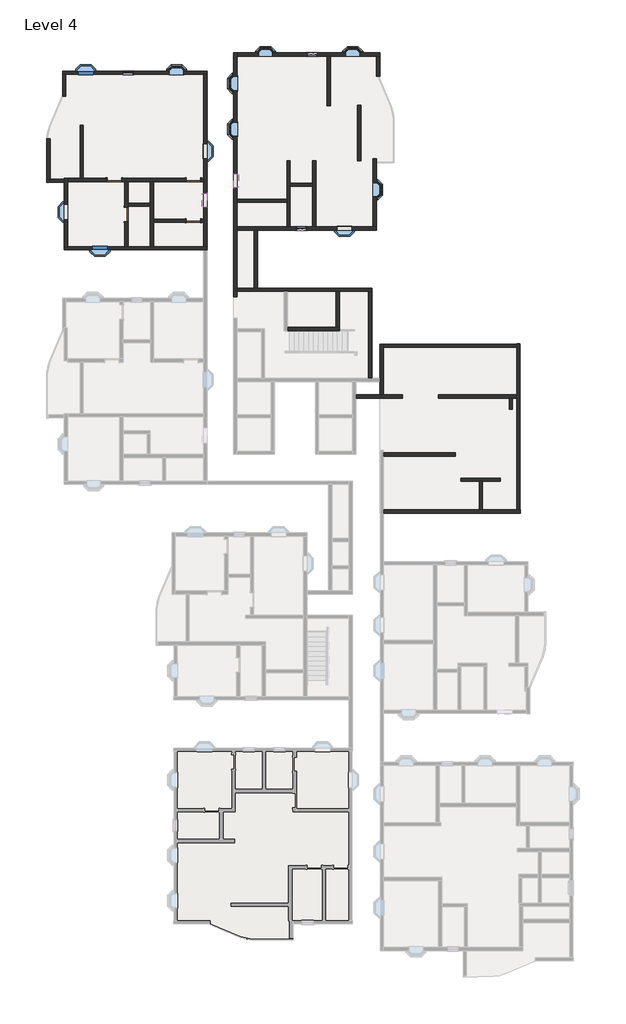
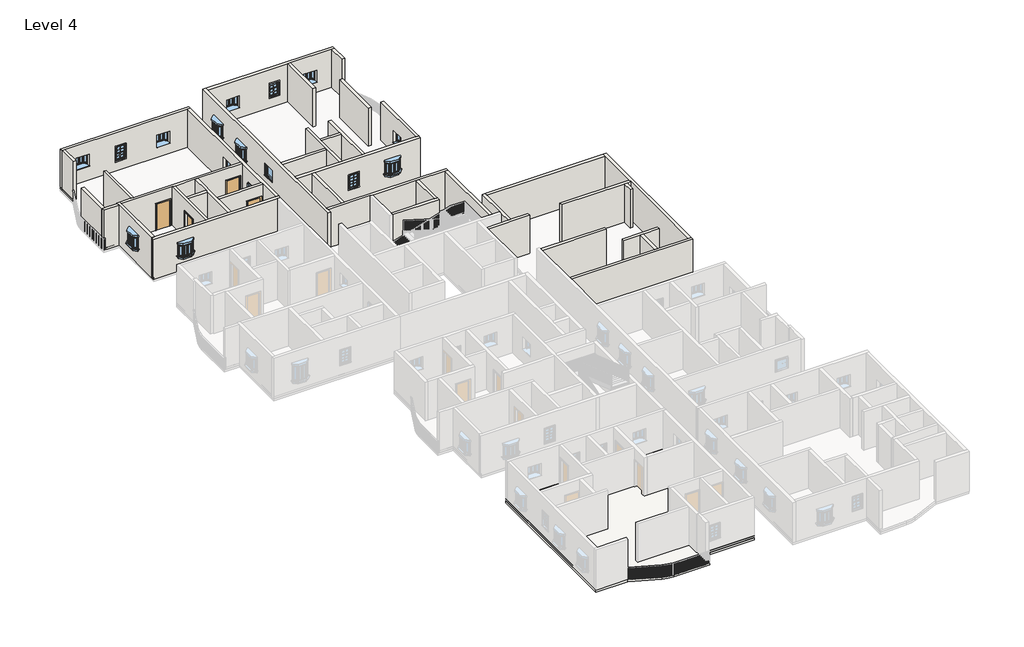
# One storey, part 4 of 14: 39 walls, 16 windows, 4 doors, 1 roof, 1 slab.
"""IFC4 building model written with IfcOpenShell, lengths in millimetres."""

from ifc_helpers import new_model, si_unit, point, frame, frame_2d, origin, place, context, project, spatial, polyline, circle_curve, trimmed, segment, composite_curve, outline, extrude, faceted_brep, transform, mapped, element, save
from components import door_719f80de, window_910x910mm_67ef725a, window_8debb0fa, windows_sgl_w_glazing_bars_910x910mm_256712d0

model = new_model("IFC4")

# Units and contexts
model_context = context("Model", 3, world=origin())
ifc_project = project(units=[si_unit("LENGTHUNIT", "METRE", prefix="MILLI")], contexts=[model_context])

# Site, building, storey
site = spatial("IfcSite", under=ifc_project)
building = spatial("IfcBuilding", under=site)
storey = spatial("IfcBuildingStorey", under=building, Name="Level 4", Elevation=9144.0)

# Doors
placement = place(None, origin())
door_shape = door_719f80de(model_context)
element("IfcDoor", 1, ObjectType="Single-Flush : 36\" x 84\"", at=placement, inside=storey, context=model_context, shape_type="MappedRepresentation", body=[
    mapped(door_shape, transform((-16068.1391351, 22048.4083494, 9144.0), x_axis=(1.0, 0.0, 0.0), y_axis=(0.0, 1.0, 0.0), z_axis=(0.0, 0.0, 1.0))),
])
element("IfcDoor", 2, ObjectType="Single-Flush : 36\" x 84\"", at=placement, inside=storey, context=model_context, shape_type="MappedRepresentation", body=[
    mapped(door_shape, transform((-15306.1391351, 19864.0083494, 9144.0), x_axis=(0.0, 1.0, 0.0), y_axis=(-1.0, 0.0, 0.0), z_axis=(0.0, 0.0, 1.0))),
])
element("IfcDoor", 3, ObjectType="Single-Flush : 36\" x 84\"", at=placement, inside=storey, context=model_context, shape_type="MappedRepresentation", body=[
    mapped(door_shape, transform((-11057.9891351, 19470.3083494, 9144.0), x_axis=(1.0, 0.0, 0.0), y_axis=(0.0, 1.0, 0.0), z_axis=(0.0, 0.0, 1.0))),
])
element("IfcDoor", 4, ObjectType="Single-Flush : 36\" x 84\"", at=placement, inside=storey, context=model_context, shape_type="MappedRepresentation", body=[
    mapped(door_shape, transform((-11057.9891351, 22048.4083494, 9144.0), x_axis=(1.0, 0.0, 0.0), y_axis=(0.0, 1.0, 0.0), z_axis=(0.0, 0.0, 1.0))),
])

# Roof
element("IfcRoof", 5, ObjectType="Generic - 12\"", at=placement, inside=storey, context=model_context, shape_type="SweptSolid", body=[
    extrude(outline(composite_curve([segment(polyline([(-10024.8708389, -25100.3416506), (-12290.487215, -25100.3416506), (-12290.487215, -13962.4416506), (-986.8891351, -13962.4416506), (-986.8891351, -25100.3416506), (-4746.0891351, -25100.3416506), (-4746.0891351, -26090.9416506), (-7315.6413127, -26090.9416506)]), True, "CONTINUOUS"), segment(trimmed(circle_curve(frame_2d((-7315.6413127, -24160.5416506)), 1930.4), [point((-7315.6413127, -26090.9416506))], [point((-8075.5356374, -25935.0851906))], False, "CARTESIAN"), True, "CONTINUOUS"), segment(polyline([(-8075.5356374, -25935.0851906), (-10024.8708389, -25100.3416506)]), True, "CONTINUOUS")], self_intersect=False)), frame((0.0, 0.0, 9144.0), z_axis=(0.0, 0.0, 1.0), x_axis=(1.0, 0.0, 0.0)), (0.0, 0.0, 1.0), 152.4),
])

# Slab
element("IfcSlab", 6, ObjectType="Generic - 12\"", at=placement, inside=storey, context=model_context, shape_type="SweptSolid", body=[
    extrude(outline(composite_curve([segment(polyline([(-10024.8708389, -25100.3416506), (-12290.487215, -25100.3416506), (-12290.487215, -13962.4416506), (-986.8891351, -13962.4416506), (-986.8891351, -25100.3416506), (-4746.0891351, -25100.3416506), (-4746.0891351, -26090.9416506), (-7315.6413127, -26090.9416506)]), True, "CONTINUOUS"), segment(trimmed(circle_curve(frame_2d((-7315.6413127, -24160.5416506)), 1930.4), [point((-7315.6413127, -26090.9416506))], [point((-8075.5356374, -25935.0851906))], False, "CARTESIAN"), True, "CONTINUOUS"), segment(polyline([(-8075.5356374, -25935.0851906), (-10024.8708389, -25100.3416506)]), True, "CONTINUOUS")], self_intersect=False)), frame((0.0, 0.0, 8991.6), z_axis=(0.0, 0.0, 1.0), x_axis=(1.0, 0.0, 0.0)), (0.0, 0.0, 1.0), 152.4),
])

# Walls
element("IfcWall", 7, ObjectType="4.5\" p", at=placement, inside=storey, context=model_context, shape_type="Brep", body=[
    faceted_brep([(-10600.7891351, 21946.8083494, 11277.6), (-10600.7891351, 21946.8083494, 9144.0), (-10397.5891351, 21946.8083494, 9144.0), (-10397.5891351, 21946.8083494, 12192.0), (-13578.9391351, 21946.8083494, 12192.0), (-13782.1391351, 21946.8083494, 12192.0), (-15204.5391351, 21946.8083494, 12192.0), (-15407.7391351, 21946.8083494, 12192.0), (-19033.5891351, 21946.8083494, 12192.0), (-19033.5891351, 21946.8083494, 9144.0), (-16525.3391351, 21946.8083494, 9144.0), (-16525.3391351, 21946.8083494, 11277.6), (-15610.9391351, 21946.8083494, 11277.6), (-15610.9391351, 21946.8083494, 9144.0), (-15407.7391351, 21946.8083494, 9144.0), (-15204.5391351, 21946.8083494, 9144.0), (-13782.1391351, 21946.8083494, 9144.0), (-13578.9391351, 21946.8083494, 9144.0), (-11515.1891351, 21946.8083494, 9144.0), (-11515.1891351, 21946.8083494, 11277.6), (-10397.5891351, 22150.0083494, 9144.0), (-10600.7891351, 22150.0083494, 9144.0), (-10600.7891351, 22150.0083494, 11277.6), (-11515.1891351, 22150.0083494, 11277.6), (-11515.1891351, 22150.0083494, 9144.0), (-15610.9391351, 22150.0083494, 9144.0), (-15610.9391351, 22150.0083494, 11277.6), (-16525.3391351, 22150.0083494, 11277.6), (-16525.3391351, 22150.0083494, 9144.0), (-18042.9891351, 22150.0083494, 9144.0), (-18246.1891351, 22150.0083494, 9144.0), (-19033.5891351, 22150.0083494, 9144.0), (-19033.5891351, 22150.0083494, 12192.0), (-18246.1891351, 22150.0083494, 12192.0), (-18042.9891351, 22150.0083494, 12192.0), (-10397.5891351, 22150.0083494, 12192.0)], [[[0, 1, 2, 3, 4, 5, 6, 7, 8, 9, 10, 11, 12, 13, 14, 15, 16, 17, 18, 19]], [[20, 21, 22, 23, 24, 25, 26, 27, 28, 29, 30, 31, 32, 33, 34, 35]], [[10, 9, 31, 30, 29, 28]], [[2, 1, 21, 20]], [[18, 17, 16, 15, 14, 13, 25, 24]], [[8, 7, 6, 5, 4, 3, 35, 34, 33, 32]], [[9, 8, 32, 31]], [[26, 25, 13, 12]], [[27, 26, 12, 11]], [[28, 27, 11, 10]], [[22, 21, 1, 0]], [[23, 22, 0, 19]], [[24, 23, 19, 18]], [[3, 2, 20, 35]]]),
])
element("IfcWall", 8, ObjectType="4.5\" p", at=placement, inside=storey, context=model_context, shape_type="Brep", body=[
    faceted_brep([(-15407.7391351, 21946.8083494, 9144.0), (-15407.7391351, 20321.2083494, 9144.0), (-15407.7391351, 20321.2083494, 11277.6), (-15407.7391351, 19406.8083494, 11277.6), (-15407.7391351, 19406.8083494, 9144.0), (-15407.7391351, 17812.9583494, 9144.0), (-15407.7391351, 17812.9583494, 12192.0), (-15407.7391351, 21946.8083494, 12192.0), (-15204.5391351, 20321.2083494, 11277.6), (-15204.5391351, 20321.2083494, 9144.0), (-15204.5391351, 20372.0083494, 9144.0), (-15204.5391351, 20575.2083494, 9144.0), (-15204.5391351, 21946.8083494, 9144.0), (-15204.5391351, 21946.8083494, 12192.0), (-15204.5391351, 20575.2083494, 12192.0), (-15204.5391351, 20372.0083494, 12192.0), (-15204.5391351, 17812.9583494, 12192.0), (-15204.5391351, 17812.9583494, 9144.0), (-15204.5391351, 19406.8083494, 9144.0), (-15204.5391351, 19406.8083494, 11277.6)], [[[0, 1, 2, 3, 4, 5, 6, 7]], [[8, 9, 10, 11, 12, 13, 14, 15, 16, 17, 18, 19]], [[18, 17, 5, 4]], [[12, 11, 10, 9, 1, 0]], [[7, 6, 16, 15, 14, 13]], [[6, 5, 17, 16]], [[0, 7, 13, 12]], [[2, 1, 9, 8]], [[3, 2, 8, 19]], [[4, 3, 19, 18]]]),
])
element("IfcWall", 9, ObjectType="4.5\" p", at=placement, inside=storey, context=model_context, shape_type="Brep", body=[
    faceted_brep([(-13782.1391351, 21946.8083494, 9144.0), (-13782.1391351, 20575.2083494, 9144.0), (-13782.1391351, 20372.0083494, 9144.0), (-13782.1391351, 17812.9583494, 9144.0), (-13782.1391351, 17812.9583494, 12192.0), (-13782.1391351, 20372.0083494, 12192.0), (-13782.1391351, 20575.2083494, 12192.0), (-13782.1391351, 21946.8083494, 12192.0), (-13578.9391351, 21946.8083494, 9144.0), (-13578.9391351, 21946.8083494, 12192.0), (-13578.9391351, 19571.9083494, 12192.0), (-13578.9391351, 19368.7083494, 12192.0), (-13578.9391351, 17812.9583494, 12192.0), (-13578.9391351, 17812.9583494, 9144.0), (-13578.9391351, 19368.7083494, 9144.0), (-13578.9391351, 19571.9083494, 9144.0)], [[[0, 1, 2, 3, 4, 5, 6, 7]], [[8, 9, 10, 11, 12, 13, 14, 15]], [[3, 2, 1, 0, 8, 15, 14, 13]], [[7, 6, 5, 4, 12, 11, 10, 9]], [[4, 3, 13, 12]], [[0, 7, 9, 8]]]),
])
element("IfcWall", 10, ObjectType="4.5\" p", at=placement, inside=storey, context=model_context, shape_type="SweptSolid", body=[
    extrude(outline(polyline([(-13782.1391351, 20372.0083494), (-15204.5391351, 20372.0083494), (-15204.5391351, 20575.2083494), (-13782.1391351, 20575.2083494), (-13782.1391351, 20372.0083494)])), frame((0.0, 0.0, 9144.0), z_axis=(0.0, 0.0, 1.0), x_axis=(1.0, 0.0, 0.0)), (0.0, 0.0, 1.0), 3048.0),
])
element("IfcWall", 11, ObjectType="4.5\" p", at=placement, inside=storey, context=model_context, shape_type="SweptSolid", body=[
    extrude(outline(polyline([(11277.6, -10600.7891351), (9144.0, -10600.7891351), (9144.0, -10397.5891351), (12192.0, -10397.5891351), (12192.0, -13578.9391351), (9144.0, -13578.9391351), (9144.0, -11515.1891351), (11277.6, -11515.1891351), (11277.6, -10600.7891351)])), frame((0.0, 19368.7083494, 0.0), z_axis=(0.0, 1.0, 0.0), x_axis=(0.0, 0.0, 1.0)), (0.0, 0.0, 1.0), 203.2),
])
element("IfcWall", 12, ObjectType="4.5\" p", at=placement, inside=storey, context=model_context, shape_type="SweptSolid", body=[
    extrude(outline(polyline([(-6993.9891351, 18875.1215905), (-6993.9891351, 15192.1215905), (-7197.1891351, 15192.1215905), (-7197.1891351, 18875.1215905), (-6993.9891351, 18875.1215905)])), frame((0.0, 0.0, 9144.0), z_axis=(0.0, 0.0, 1.0), x_axis=(1.0, 0.0, 0.0)), (0.0, 0.0, 1.0), 3048.0),
])
element("IfcWall", 13, ObjectType="4.5\" p", at=placement, inside=storey, context=model_context, shape_type="Brep", body=[
    faceted_brep([(-8289.3891351, 18875.1215905, 9144.0), (-7197.1891351, 18875.1215905, 9144.0), (-6993.9891351, 18875.1215905, 9144.0), (562.5108649, 18875.1215905, 9144.0), (562.5108649, 18875.1215905, 12192.0), (-6993.9891351, 18875.1215905, 12192.0), (-7197.1891351, 18875.1215905, 12192.0), (-8289.3891351, 18875.1215905, 12192.0), (-1017.6641351, 18875.1215905, 11254.0), (-1017.6641351, 18875.1215905, 10344.0), (-1927.6641351, 18875.1215905, 10344.0), (-1927.6641351, 18875.1215905, 11254.0), (-3876.1391351, 18875.1215905, 11125.2), (-3876.1391351, 18875.1215905, 10058.4), (-4536.5391351, 18875.1215905, 10058.4), (-4536.5391351, 18875.1215905, 11125.2), (-8289.3891351, 19078.3215905, 9144.0), (-8289.3891351, 19078.3215905, 12192.0), (-5120.7391351, 19078.3215905, 12192.0), (-4917.5391351, 19078.3215905, 12192.0), (-3495.1391351, 19078.3215905, 12192.0), (-3291.9391351, 19078.3215905, 12192.0), (346.6108649, 19078.3215905, 12192.0), (549.8108649, 19078.3215905, 12192.0), (562.5108649, 19078.3215905, 12192.0), (562.5108649, 19078.3215905, 9144.0), (549.8108649, 19078.3215905, 9144.0), (346.6108649, 19078.3215905, 9144.0), (-3291.9391351, 19078.3215905, 9144.0), (-3495.1391351, 19078.3215905, 9144.0), (-4917.5391351, 19078.3215905, 9144.0), (-5120.7391351, 19078.3215905, 9144.0), (-1017.6641351, 19078.3215905, 11254.0), (-1927.6641351, 19078.3215905, 11254.0), (-1927.6641351, 19078.3215905, 10344.0), (-1017.6641351, 19078.3215905, 10344.0), (-3876.1391351, 19078.3215905, 11125.2), (-4536.5391351, 19078.3215905, 11125.2), (-4536.5391351, 19078.3215905, 10058.4), (-3876.1391351, 19078.3215905, 10058.4)], [[[0, 1, 2, 3, 4, 5, 6, 7], [8, 9, 10, 11], [12, 13, 14, 15]], [[16, 17, 18, 19, 20, 21, 22, 23, 24, 25, 26, 27, 28, 29, 30, 31], [32, 33, 34, 35], [36, 37, 38, 39]], [[3, 2, 1, 0, 16, 31, 30, 29, 28, 27, 26, 25]], [[4, 3, 25, 24]], [[7, 6, 5, 4, 24, 23, 22, 21, 20, 19, 18, 17]], [[9, 8, 32, 35]], [[10, 9, 35, 34]], [[11, 10, 34, 33]], [[8, 11, 33, 32]], [[13, 12, 36, 39]], [[14, 13, 39, 38]], [[15, 14, 38, 37]], [[12, 15, 37, 36]], [[0, 7, 17, 16]]]),
])
element("IfcWall", 14, ObjectType="4.5\" p", at=placement, inside=storey, context=model_context, shape_type="SweptSolid", body=[
    extrude(outline(polyline([(19078.3215905, 9144.0), (19078.3215905, 12192.0), (23396.3215905, 12192.0), (23396.3215905, 9144.0), (19078.3215905, 9144.0)]), holes=[polyline([(21882.8215905, 10968.4), (20972.8215905, 10968.4), (20972.8215905, 10058.4), (21882.8215905, 10058.4), (21882.8215905, 10968.4)])]), frame((346.6108649, 0.0, 0.0), z_axis=(1.0, 0.0, 0.0), x_axis=(0.0, 1.0, 0.0)), (0.0, 0.0, 1.0), 203.2),
])
element("IfcWall", 15, ObjectType="4.5\" p", at=placement, inside=storey, context=model_context, shape_type="SweptSolid", body=[
    extrude(outline(polyline([(-5120.7391351, 20634.0715905), (-8289.3891351, 20634.0715905), (-8289.3891351, 20837.2715905), (-5120.7391351, 20837.2715905), (-5120.7391351, 20634.0715905)])), frame((0.0, 0.0, 9144.0), z_axis=(0.0, 0.0, 1.0), x_axis=(1.0, 0.0, 0.0)), (0.0, 0.0, 1.0), 3048.0),
])
element("IfcWall", 16, ObjectType="4.5\" p", at=placement, inside=storey, context=model_context, shape_type="Brep", body=[
    faceted_brep([(-5120.7391351, 23256.6215905, 9144.0), (-5120.7391351, 20837.2715905, 9144.0), (-5120.7391351, 20634.0715905, 9144.0), (-5120.7391351, 19078.3215905, 9144.0), (-5120.7391351, 19078.3215905, 12192.0), (-5120.7391351, 20634.0715905, 12192.0), (-5120.7391351, 20837.2715905, 12192.0), (-5120.7391351, 23256.6215905, 12192.0), (-4917.5391351, 23256.6215905, 9144.0), (-4917.5391351, 23256.6215905, 12192.0), (-4917.5391351, 21853.2715905, 12192.0), (-4917.5391351, 21650.0715905, 12192.0), (-4917.5391351, 19078.3215905, 12192.0), (-4917.5391351, 19078.3215905, 9144.0), (-4917.5391351, 21650.0715905, 9144.0), (-4917.5391351, 21853.2715905, 9144.0)], [[[0, 1, 2, 3, 4, 5, 6, 7]], [[8, 9, 10, 11, 12, 13, 14, 15]], [[3, 2, 1, 0, 8, 15, 14, 13]], [[7, 6, 5, 4, 12, 11, 10, 9]], [[0, 7, 9, 8]], [[4, 3, 13, 12]]]),
])
element("IfcWall", 17, ObjectType="4.5\" p", at=placement, inside=storey, context=model_context, shape_type="Brep", body=[
    faceted_brep([(-3495.1391351, 23256.6215905, 9144.0), (-3495.1391351, 21853.2715905, 9144.0), (-3495.1391351, 21650.0715905, 9144.0), (-3495.1391351, 19078.3215905, 9144.0), (-3495.1391351, 19078.3215905, 12192.0), (-3495.1391351, 21650.0715905, 12192.0), (-3495.1391351, 21853.2715905, 12192.0), (-3495.1391351, 23256.6215905, 12192.0), (-3291.9391351, 23256.6215905, 9144.0), (-3291.9391351, 23256.6215905, 12192.0), (-3291.9391351, 19078.3215905, 12192.0), (-3291.9391351, 19078.3215905, 9144.0)], [[[0, 1, 2, 3, 4, 5, 6, 7]], [[8, 9, 10, 11]], [[3, 2, 1, 0, 8, 11]], [[7, 6, 5, 4, 10, 9]], [[0, 7, 9, 8]], [[4, 3, 11, 10]]]),
])
element("IfcWall", 18, ObjectType="4.5\" p", at=placement, inside=storey, context=model_context, shape_type="SweptSolid", body=[
    extrude(outline(polyline([(-3495.1391351, 21650.0715905), (-4917.5391351, 21650.0715905), (-4917.5391351, 21853.2715905), (-3495.1391351, 21853.2715905), (-3495.1391351, 21650.0715905)])), frame((0.0, 0.0, 9144.0), z_axis=(0.0, 0.0, 1.0), x_axis=(1.0, 0.0, 0.0)), (0.0, 0.0, 1.0), 3048.0),
])
element("IfcWall", 19, ObjectType="4.5\" p", at=placement, inside=storey, context=model_context, shape_type="SweptSolid", body=[
    extrude(outline(polyline([(-1799.6891351, 14988.9215905), (-1799.6891351, 12709.2715905), (-2002.8891351, 12709.2715905), (-2002.8891351, 14988.9215905), (-1799.6891351, 14988.9215905)])), frame((0.0, 0.0, 9144.0), z_axis=(0.0, 0.0, 1.0), x_axis=(1.0, 0.0, 0.0)), (0.0, 0.0, 1.0), 3048.0),
])
element("IfcWall", 20, ObjectType="4.5\" p", at=placement, inside=storey, context=model_context, shape_type="Brep", body=[
    faceted_brep([(-5095.3391351, 12506.0715905, 9144.0), (-1786.9891351, 12506.0715905, 9144.0), (-1786.9891351, 12506.0715905, 12192.0), (-5095.3391351, 12506.0715905, 12192.0), (-5095.3391351, 12709.2715905, 9144.0), (-5095.3391351, 12709.2715905, 12192.0), (-2002.8891351, 12709.2715905, 12192.0), (-1799.6891351, 12709.2715905, 12192.0), (-1786.9891351, 12709.2715905, 12192.0), (-1786.9891351, 12709.2715905, 9144.0), (-1799.6891351, 12709.2715905, 9144.0), (-2002.8891351, 12709.2715905, 9144.0)], [[[0, 1, 2, 3]], [[4, 5, 6, 7, 8, 9, 10, 11]], [[1, 0, 4, 11, 10, 9]], [[2, 1, 9, 8]], [[3, 2, 8, 7, 6, 5]], [[0, 3, 5, 4]]]),
])
element("IfcWall", 21, ObjectType="4.5\" p", at=placement, inside=storey, context=model_context, shape_type="Brep", body=[
    faceted_brep([(-745.5891351, 8223.6457306, 9144.0), (2209.4205024, 8223.6457306, 9144.0), (2209.4205024, 8223.6457306, 12192.0), (-745.5891351, 8223.6457306, 12192.0), (-745.5891351, 8426.8457306, 9144.0), (-745.5891351, 8426.8457306, 12192.0), (793.5880523, 8426.8457306, 12192.0), (996.7880523, 8426.8457306, 12192.0), (2209.4205024, 8426.8457306, 12192.0), (2209.4205024, 8426.8457306, 9144.0), (996.7880523, 8426.8457306, 9144.0), (793.5880523, 8426.8457306, 9144.0)], [[[0, 1, 2, 3]], [[4, 5, 6, 7, 8, 9, 10, 11]], [[1, 0, 4, 11, 10, 9]], [[2, 1, 9, 8]], [[3, 2, 8, 7, 6, 5]], [[0, 3, 5, 4]]]),
])
element("IfcWall", 22, ObjectType="4.5\" p", at=placement, inside=storey, context=model_context, shape_type="Brep", body=[
    faceted_brep([(996.7880523, 8426.8457306, 9144.0), (996.7880523, 11443.0957306, 9144.0), (996.7880523, 11646.2957306, 9144.0), (996.7880523, 11646.2957306, 12192.0), (996.7880523, 11443.0957306, 12192.0), (996.7880523, 8426.8457306, 12192.0), (793.5880523, 8426.8457306, 9144.0), (793.5880523, 8426.8457306, 12192.0), (793.5880523, 9275.2949943, 12192.0), (793.5880523, 9478.4949943, 12192.0), (793.5880523, 11646.2957306, 12192.0), (793.5880523, 11646.2957306, 9144.0), (793.5880523, 9478.4949943, 9144.0), (793.5880523, 9275.2949943, 9144.0)], [[[0, 1, 2, 3, 4, 5]], [[6, 7, 8, 9, 10, 11, 12, 13]], [[2, 1, 0, 6, 13, 12, 11]], [[5, 4, 3, 10, 9, 8, 7]], [[0, 5, 7, 6]], [[3, 2, 11, 10]]]),
])
element("IfcWall", 23, ObjectType="4.5\" p", at=placement, inside=storey, context=model_context, shape_type="Brep", body=[
    faceted_brep([(9461.3380523, 8426.8457306, 9144.0), (4492.3034266, 8426.8457306, 9144.0), (4492.3034266, 8426.8457306, 12192.0), (9461.3380523, 8426.8457306, 12192.0), (9461.3380523, 8223.6457306, 9144.0), (9461.3380523, 8223.6457306, 12192.0), (9181.9380523, 8223.6457306, 12192.0), (8978.7380523, 8223.6457306, 12192.0), (4492.3034266, 8223.6457306, 12192.0), (4492.3034266, 8223.6457306, 9144.0), (8978.7380523, 8223.6457306, 9144.0), (9181.9380523, 8223.6457306, 9144.0)], [[[0, 1, 2, 3]], [[4, 5, 6, 7, 8, 9, 10, 11]], [[1, 0, 4, 11, 10, 9]], [[2, 1, 9, 8]], [[3, 2, 8, 7, 6, 5]], [[0, 3, 5, 4]]]),
])
element("IfcWall", 24, ObjectType="4.5\" p", at=placement, inside=storey, context=model_context, shape_type="Brep", body=[
    faceted_brep([(1007.0108649, 940.1957306, 9144.0), (9677.2380523, 940.1957306, 9144.0), (9677.2380523, 940.1957306, 12192.0), (1007.0108649, 940.1957306, 12192.0), (1007.0108649, 1143.3957306, 9144.0), (1007.0108649, 1143.3957306, 12192.0), (7073.7380523, 1143.3957306, 12192.0), (7276.9380523, 1143.3957306, 12192.0), (9461.3380523, 1143.3957306, 12192.0), (9664.5380523, 1143.3957306, 12192.0), (9677.2380523, 1143.3957306, 12192.0), (9677.2380523, 1143.3957306, 9144.0), (9664.5380523, 1143.3957306, 9144.0), (9461.3380523, 1143.3957306, 9144.0), (7276.9380523, 1143.3957306, 9144.0), (7073.7380523, 1143.3957306, 9144.0)], [[[0, 1, 2, 3]], [[4, 5, 6, 7, 8, 9, 10, 11, 12, 13, 14, 15]], [[1, 0, 4, 15, 14, 13, 12, 11]], [[2, 1, 11, 10]], [[3, 2, 10, 9, 8, 7, 6, 5]], [[0, 3, 5, 4]]]),
])
element("IfcWall", 25, ObjectType="4.5\" p", at=placement, inside=storey, context=model_context, shape_type="Brep", body=[
    faceted_brep([(9664.5380523, 1143.3957306, 9144.0), (9664.5380523, 11658.9957306, 9144.0), (9664.5380523, 11658.9957306, 12192.0), (9664.5380523, 1143.3957306, 12192.0), (9461.3380523, 1143.3957306, 9144.0), (9461.3380523, 1143.3957306, 12192.0), (9461.3380523, 8223.6457306, 12192.0), (9461.3380523, 8426.8457306, 12192.0), (9461.3380523, 11443.0957306, 12192.0), (9461.3380523, 11646.2957306, 12192.0), (9461.3380523, 11658.9957306, 12192.0), (9461.3380523, 11658.9957306, 9144.0), (9461.3380523, 11646.2957306, 9144.0), (9461.3380523, 11443.0957306, 9144.0), (9461.3380523, 8426.8457306, 9144.0), (9461.3380523, 8223.6457306, 9144.0)], [[[0, 1, 2, 3]], [[4, 5, 6, 7, 8, 9, 10, 11, 12, 13, 14, 15]], [[1, 0, 4, 15, 14, 13, 12, 11]], [[2, 1, 11, 10]], [[3, 2, 10, 9, 8, 7, 6, 5]], [[0, 3, 5, 4]]]),
])
element("IfcWall", 26, ObjectType="4.5\" p", at=placement, inside=storey, context=model_context, shape_type="SweptSolid", body=[
    extrude(outline(polyline([(-18246.1891351, 22150.0083494), (-18246.1891351, 25515.5083494), (-18042.9891351, 25515.5083494), (-18042.9891351, 22150.0083494), (-18246.1891351, 22150.0083494)])), frame((0.0, 0.0, 9144.0), z_axis=(0.0, 0.0, 1.0), x_axis=(1.0, 0.0, 0.0)), (0.0, 0.0, 1.0), 3048.0),
])
element("IfcWall", 27, ObjectType="4.5\" p", at=placement, inside=storey, context=model_context, shape_type="SweptSolid", body=[
    extrude(outline(polyline([(-643.9891351, 23256.6215905), (-643.9891351, 26780.8715905), (-440.7891351, 26780.8715905), (-440.7891351, 23256.6215905), (-643.9891351, 23256.6215905)])), frame((0.0, 0.0, 9144.0), z_axis=(0.0, 0.0, 1.0), x_axis=(1.0, 0.0, 0.0)), (0.0, 0.0, 1.0), 3048.0),
])
element("IfcWall", 28, ObjectType="4.5\" p", at=placement, inside=storey, context=model_context, shape_type="SweptSolid", body=[
    extrude(outline(polyline([(-2568.0391351, 26760.9286213), (-2568.0391351, 29898.7215905), (-2364.8391351, 29898.7215905), (-2364.8391351, 26760.9286213), (-2568.0391351, 26760.9286213)])), frame((0.0, 0.0, 9144.0), z_axis=(0.0, 0.0, 1.0), x_axis=(1.0, 0.0, 0.0)), (0.0, 0.0, 1.0), 3048.0),
])
element("IfcWall", 29, ObjectType="4.5\" p", at=placement, inside=storey, context=model_context, shape_type="SweptSolid", body=[
    extrude(outline(polyline([(765.7108649, 29898.7215905), (765.7108649, 28631.1875845), (562.5108649, 28631.1875845), (562.5108649, 29898.7215905), (765.7108649, 29898.7215905)])), frame((0.0, 0.0, 9144.0), z_axis=(0.0, 0.0, 1.0), x_axis=(1.0, 0.0, 0.0)), (0.0, 0.0, 1.0), 3048.0),
])
element("IfcWall", 30, ObjectType="9\" w", at=placement, inside=storey, context=model_context, shape_type="Brep", body=[
    faceted_brep([(-10181.6891351, 17812.9583494, 9144.0), (-10194.3891351, 17812.9583494, 9144.0), (-10397.5891351, 17812.9583494, 9144.0), (-13578.9391351, 17812.9583494, 9144.0), (-13782.1391351, 17812.9583494, 9144.0), (-15204.5391351, 17812.9583494, 9144.0), (-15407.7391351, 17812.9583494, 9144.0), (-19033.5891351, 17812.9583494, 9144.0), (-19236.7891351, 17812.9583494, 9144.0), (-19249.4891351, 17812.9583494, 9144.0), (-19249.4891351, 17812.9583494, 12192.0), (-19236.7891351, 17812.9583494, 12192.0), (-19033.5891351, 17812.9583494, 12192.0), (-15407.7391351, 17812.9583494, 12192.0), (-15204.5391351, 17812.9583494, 12192.0), (-13782.1391351, 17812.9583494, 12192.0), (-13578.9391351, 17812.9583494, 12192.0), (-10397.5891351, 17812.9583494, 12192.0), (-10194.3891351, 17812.9583494, 12192.0), (-10181.6891351, 17812.9583494, 12192.0), (-16527.5391351, 17812.9583494, 11254.0), (-17437.5391351, 17812.9583494, 11254.0), (-17437.5391351, 17812.9583494, 10344.0), (-16527.5391351, 17812.9583494, 10344.0), (-10181.6891351, 17609.7583494, 9144.0), (-10181.6891351, 17609.7583494, 12192.0), (-19249.4891351, 17609.7583494, 12192.0), (-19249.4891351, 17609.7583494, 9144.0), (-16527.5391351, 17609.7583494, 11254.0), (-16527.5391351, 17609.7583494, 10344.0), (-17437.5391351, 17609.7583494, 10344.0), (-17437.5391351, 17609.7583494, 11254.0)], [[[0, 1, 2, 3, 4, 5, 6, 7, 8, 9, 10, 11, 12, 13, 14, 15, 16, 17, 18, 19], [20, 21, 22, 23]], [[24, 25, 26, 27], [28, 29, 30, 31]], [[9, 8, 7, 6, 5, 4, 3, 2, 1, 0, 24, 27]], [[10, 9, 27, 26]], [[19, 18, 17, 16, 15, 14, 13, 12, 11, 10, 26, 25]], [[0, 19, 25, 24]], [[29, 28, 20, 23]], [[30, 29, 23, 22]], [[31, 30, 22, 21]], [[28, 31, 21, 20]]]),
])
element("IfcWall", 31, ObjectType="9\" w", at=placement, inside=storey, context=model_context, shape_type="Brep", body=[
    faceted_brep([(-19033.5891351, 17812.9583494, 9144.0), (-19033.5891351, 21946.8083494, 9144.0), (-19033.5891351, 22150.0083494, 9144.0), (-19033.5891351, 22150.0083494, 12192.0), (-19033.5891351, 21946.8083494, 12192.0), (-19033.5891351, 17812.9583494, 12192.0), (-19033.5891351, 19555.0583494, 11254.0), (-19033.5891351, 20465.0583494, 11254.0), (-19033.5891351, 20465.0583494, 10344.0), (-19033.5891351, 19555.0583494, 10344.0), (-19236.7891351, 17812.9583494, 9144.0), (-19236.7891351, 17812.9583494, 12192.0), (-19236.7891351, 21889.6583494, 12192.0), (-19236.7891351, 22092.8583494, 12192.0), (-19236.7891351, 22150.0083494, 12192.0), (-19236.7891351, 22150.0083494, 9144.0), (-19236.7891351, 22092.8583494, 9144.0), (-19236.7891351, 21889.6583494, 9144.0), (-19236.7891351, 19555.0583494, 11254.0), (-19236.7891351, 19555.0583494, 10344.0), (-19236.7891351, 20465.0583494, 10344.0), (-19236.7891351, 20465.0583494, 11254.0)], [[[0, 1, 2, 3, 4, 5], [6, 7, 8, 9]], [[10, 11, 12, 13, 14, 15, 16, 17], [18, 19, 20, 21]], [[2, 1, 0, 10, 17, 16, 15]], [[5, 4, 3, 14, 13, 12, 11]], [[0, 5, 11, 10]], [[3, 2, 15, 14]], [[19, 18, 6, 9]], [[20, 19, 9, 8]], [[21, 20, 8, 7]], [[18, 21, 7, 6]]]),
])
element("IfcWall", 32, ObjectType="9\" w", at=placement, inside=storey, context=model_context, shape_type="Brep", body=[
    faceted_brep([(-20341.6891351, 21889.6583494, 9144.0), (-19236.7891351, 21889.6583494, 9144.0), (-19236.7891351, 21889.6583494, 12192.0), (-20341.6891351, 21889.6583494, 12192.0), (-20341.6891351, 22092.8583494, 9144.0), (-20341.6891351, 22092.8583494, 12192.0), (-20138.4891351, 22092.8583494, 12192.0), (-19236.7891351, 22092.8583494, 12192.0), (-19236.7891351, 22092.8583494, 9144.0), (-20138.4891351, 22092.8583494, 9144.0)], [[[0, 1, 2, 3]], [[4, 5, 6, 7, 8, 9]], [[1, 0, 4, 9, 8]], [[3, 2, 7, 6, 5]], [[0, 3, 5, 4]], [[2, 1, 8, 7]]]),
])
element("IfcWall", 33, ObjectType="9\" w", at=placement, inside=storey, context=model_context, shape_type="SweptSolid", body=[
    extrude(outline(polyline([(-20341.6891351, 22092.8583494), (-20341.6891351, 24656.5948172), (-20138.4891351, 24656.5948172), (-20138.4891351, 22092.8583494), (-20341.6891351, 22092.8583494)])), frame((0.0, 0.0, 9144.0), z_axis=(0.0, 0.0, 1.0), x_axis=(1.0, 0.0, 0.0)), (0.0, 0.0, 1.0), 3048.0),
])
element("IfcWall", 34, ObjectType="9\" w", at=placement, inside=storey, context=model_context, shape_type="Brep", body=[
    faceted_brep([(-8289.3891351, 14988.9215905, 9144.0), (-5298.5391351, 14988.9215905, 9144.0), (-5095.3391351, 14988.9215905, 9144.0), (-2002.8891351, 14988.9215905, 9144.0), (-1799.6891351, 14988.9215905, 9144.0), (54.5108649, 14988.9215905, 9144.0), (257.7108649, 14988.9215905, 9144.0), (270.4108649, 14988.9215905, 9144.0), (270.4108649, 14988.9215905, 12192.0), (257.7108649, 14988.9215905, 12192.0), (54.5108649, 14988.9215905, 12192.0), (-1799.6891351, 14988.9215905, 12192.0), (-2002.8891351, 14988.9215905, 12192.0), (-5095.3391351, 14988.9215905, 12192.0), (-5298.5391351, 14988.9215905, 12192.0), (-8289.3891351, 14988.9215905, 12192.0), (-8289.3891351, 15192.1215905, 9144.0), (-8289.3891351, 15192.1215905, 12192.0), (-7197.1891351, 15192.1215905, 12192.0), (-6993.9891351, 15192.1215905, 12192.0), (270.4108649, 15192.1215905, 12192.0), (270.4108649, 15192.1215905, 9144.0), (-6993.9891351, 15192.1215905, 9144.0), (-7197.1891351, 15192.1215905, 9144.0)], [[[0, 1, 2, 3, 4, 5, 6, 7, 8, 9, 10, 11, 12, 13, 14, 15]], [[16, 17, 18, 19, 20, 21, 22, 23]], [[7, 6, 5, 4, 3, 2, 1, 0, 16, 23, 22, 21]], [[8, 7, 21, 20]], [[15, 14, 13, 12, 11, 10, 9, 8, 20, 19, 18, 17]], [[0, 15, 17, 16]]]),
])
element("IfcWall", 35, ObjectType="9\" w", at=placement, inside=storey, context=model_context, shape_type="SweptSolid", body=[
    extrude(outline(polyline([(54.5108649, 9478.4949943), (54.5108649, 14988.9215905), (257.7108649, 14988.9215905), (257.7108649, 9478.4949943), (54.5108649, 9478.4949943)])), frame((0.0, 0.0, 9144.0), z_axis=(0.0, 0.0, 1.0), x_axis=(1.0, 0.0, 0.0)), (0.0, 0.0, 1.0), 3048.0),
])
element("IfcWall", 36, ObjectType="9\" w", at=placement, inside=storey, context=model_context, shape_type="SweptSolid", body=[
    extrude(outline(polyline([(9461.3380523, 11443.0957306), (996.7880523, 11443.0957306), (996.7880523, 11646.2957306), (9461.3380523, 11646.2957306), (9461.3380523, 11443.0957306)])), frame((0.0, 0.0, 9144.0), z_axis=(0.0, 0.0, 1.0), x_axis=(1.0, 0.0, 0.0)), (0.0, 0.0, 1.0), 3048.0),
])
element("IfcWall", 37, ObjectType="9\" w", at=placement, inside=storey, context=model_context, shape_type="SweptSolid", body=[
    extrude(outline(polyline([(8978.7380523, 7506.0957306), (8978.7380523, 8223.6457306), (9181.9380523, 8223.6457306), (9181.9380523, 7506.0957306), (8978.7380523, 7506.0957306)])), frame((0.0, 0.0, 9144.0), z_axis=(0.0, 0.0, 1.0), x_axis=(1.0, 0.0, 0.0)), (0.0, 0.0, 1.0), 3048.0),
])
element("IfcWall", 38, ObjectType="9\" w", at=placement, inside=storey, context=model_context, shape_type="SweptSolid", body=[
    extrude(outline(polyline([(7276.9380523, 2954.8622042), (7276.9380523, 1143.3957306), (7073.7380523, 1143.3957306), (7073.7380523, 2954.8622042), (7276.9380523, 2954.8622042)])), frame((0.0, 0.0, 9144.0), z_axis=(0.0, 0.0, 1.0), x_axis=(1.0, 0.0, 0.0)), (0.0, 0.0, 1.0), 3048.0),
])
element("IfcWall", 39, ObjectType="9\" w", at=placement, inside=storey, context=model_context, shape_type="Brep", body=[
    faceted_brep([(5904.1857655, 2954.8622042, 9144.0), (7073.7380523, 2954.8622042, 9144.0), (7276.9380523, 2954.8622042, 9144.0), (8418.7857655, 2954.8622042, 9144.0), (8418.7857655, 2954.8622042, 12192.0), (7276.9380523, 2954.8622042, 12192.0), (7073.7380523, 2954.8622042, 12192.0), (5904.1857655, 2954.8622042, 12192.0), (5904.1857655, 3158.0622042, 9144.0), (5904.1857655, 3158.0622042, 12192.0), (8418.7857655, 3158.0622042, 12192.0), (8418.7857655, 3158.0622042, 9144.0)], [[[0, 1, 2, 3, 4, 5, 6, 7]], [[8, 9, 10, 11]], [[3, 2, 1, 0, 8, 11]], [[4, 3, 11, 10]], [[7, 6, 5, 4, 10, 9]], [[0, 7, 9, 8]]]),
])
element("IfcWall", 40, ObjectType="9\" w", at=placement, inside=storey, context=model_context, shape_type="SweptSolid", body=[
    extrude(outline(polyline([(5571.3060189, 4550.8949943), (1007.0108649, 4550.8949943), (1007.0108649, 4754.0949943), (5571.3060189, 4754.0949943), (5571.3060189, 4550.8949943)])), frame((0.0, 0.0, 9144.0), z_axis=(0.0, 0.0, 1.0), x_axis=(1.0, 0.0, 0.0)), (0.0, 0.0, 1.0), 3048.0),
])
element("IfcWall", 41, ObjectType="9\" w", at=placement, inside=storey, context=model_context, shape_type="Brep", body=[
    faceted_brep([(-8390.9891351, 29898.7215905, 9144.0), (-2568.0391351, 29898.7215905, 9144.0), (-2364.8391351, 29898.7215905, 9144.0), (562.5108649, 29898.7215905, 9144.0), (765.7108649, 29898.7215905, 9144.0), (765.7108649, 29898.7215905, 12192.0), (562.5108649, 29898.7215905, 12192.0), (-2364.8391351, 29898.7215905, 12192.0), (-2568.0391351, 29898.7215905, 12192.0), (-8390.9891351, 29898.7215905, 12192.0), (-6931.4641351, 29898.7215905, 10968.4), (-6021.4641351, 29898.7215905, 10968.4), (-6021.4641351, 29898.7215905, 10058.4), (-6931.4641351, 29898.7215905, 10058.4), (-1406.9641351, 29898.7215905, 10968.4), (-496.9641351, 29898.7215905, 10968.4), (-496.9641351, 29898.7215905, 10058.4), (-1406.9641351, 29898.7215905, 10058.4), (-3844.3891351, 29898.7215905, 11125.2), (-3183.9891351, 29898.7215905, 11125.2), (-3183.9891351, 29898.7215905, 10058.4), (-3844.3891351, 29898.7215905, 10058.4), (-8390.9891351, 30101.9215905, 9144.0), (-8390.9891351, 30101.9215905, 12192.0), (765.7108649, 30101.9215905, 12192.0), (765.7108649, 30101.9215905, 9144.0), (-6931.4641351, 30101.9215905, 10968.4), (-6931.4641351, 30101.9215905, 10058.4), (-6021.4641351, 30101.9215905, 10058.4), (-6021.4641351, 30101.9215905, 10968.4), (-1406.9641351, 30101.9215905, 10968.4), (-1406.9641351, 30101.9215905, 10058.4), (-496.9641351, 30101.9215905, 10058.4), (-496.9641351, 30101.9215905, 10968.4), (-3844.3891351, 30101.9215905, 11125.2), (-3844.3891351, 30101.9215905, 10058.4), (-3183.9891351, 30101.9215905, 10058.4), (-3183.9891351, 30101.9215905, 11125.2)], [[[0, 1, 2, 3, 4, 5, 6, 7, 8, 9], [10, 11, 12, 13], [14, 15, 16, 17], [18, 19, 20, 21]], [[22, 23, 24, 25], [26, 27, 28, 29], [30, 31, 32, 33], [34, 35, 36, 37]], [[4, 3, 2, 1, 0, 22, 25]], [[9, 8, 7, 6, 5, 24, 23]], [[0, 9, 23, 22]], [[27, 26, 10, 13]], [[28, 27, 13, 12]], [[29, 28, 12, 11]], [[26, 29, 11, 10]], [[31, 30, 14, 17]], [[32, 31, 17, 16]], [[33, 32, 16, 15]], [[30, 33, 15, 14]], [[35, 34, 18, 21]], [[36, 35, 21, 20]], [[37, 36, 20, 19]], [[34, 37, 19, 18]], [[5, 4, 25, 24]]]),
])
element("IfcWall", 42, ObjectType="9\" w", at=placement, inside=storey, context=model_context, shape_type="Brep", body=[
    faceted_brep([(-19351.0891351, 28747.6583494, 9144.0), (-19147.8891351, 28747.6583494, 9144.0), (-10397.5891351, 28747.6583494, 9144.0), (-10194.3891351, 28747.6583494, 9144.0), (-10181.6891351, 28747.6583494, 9144.0), (-10181.6891351, 28747.6583494, 12192.0), (-10194.3891351, 28747.6583494, 12192.0), (-10397.5891351, 28747.6583494, 12192.0), (-19147.8891351, 28747.6583494, 12192.0), (-19351.0891351, 28747.6583494, 12192.0), (-18332.8891351, 28747.6583494, 11254.0), (-17422.8891351, 28747.6583494, 11254.0), (-17422.8891351, 28747.6583494, 10344.0), (-18332.8891351, 28747.6583494, 10344.0), (-12579.7891351, 28747.6583494, 10968.4), (-11669.7891351, 28747.6583494, 10968.4), (-11669.7891351, 28747.6583494, 10058.4), (-12579.7891351, 28747.6583494, 10058.4), (-14845.7641351, 28747.6583494, 11125.2), (-14845.7641351, 28747.6583494, 10058.4), (-15506.1641351, 28747.6583494, 10058.4), (-15506.1641351, 28747.6583494, 11125.2), (-19351.0891351, 28950.8583494, 9144.0), (-19351.0891351, 28950.8583494, 12192.0), (-10181.6891351, 28950.8583494, 12192.0), (-10181.6891351, 28950.8583494, 9144.0), (-18332.8891351, 28950.8583494, 11254.0), (-18332.8891351, 28950.8583494, 10344.0), (-17422.8891351, 28950.8583494, 10344.0), (-17422.8891351, 28950.8583494, 11254.0), (-12579.7891351, 28950.8583494, 10968.4), (-12579.7891351, 28950.8583494, 10058.4), (-11669.7891351, 28950.8583494, 10058.4), (-11669.7891351, 28950.8583494, 10968.4), (-14845.7641351, 28950.8583494, 11125.2), (-15506.1641351, 28950.8583494, 11125.2), (-15506.1641351, 28950.8583494, 10058.4), (-14845.7641351, 28950.8583494, 10058.4)], [[[0, 1, 2, 3, 4, 5, 6, 7, 8, 9], [10, 11, 12, 13], [14, 15, 16, 17], [18, 19, 20, 21]], [[22, 23, 24, 25], [26, 27, 28, 29], [30, 31, 32, 33], [34, 35, 36, 37]], [[4, 3, 2, 1, 0, 22, 25]], [[5, 4, 25, 24]], [[9, 8, 7, 6, 5, 24, 23]], [[27, 26, 10, 13]], [[28, 27, 13, 12]], [[29, 28, 12, 11]], [[26, 29, 11, 10]], [[31, 30, 14, 17]], [[32, 31, 17, 16]], [[33, 32, 16, 15]], [[30, 33, 15, 14]], [[19, 18, 34, 37]], [[20, 19, 37, 36]], [[21, 20, 36, 35]], [[18, 21, 35, 34]], [[0, 9, 23, 22]]]),
])
element("IfcWall", 43, ObjectType="9\" w", at=placement, inside=storey, context=model_context, shape_type="SweptSolid", body=[
    extrude(outline(polyline([(-19147.8891351, 28747.6583494), (-19147.8891351, 27344.9858981), (-19351.0891351, 27344.9858981), (-19351.0891351, 28747.6583494), (-19147.8891351, 28747.6583494)])), frame((0.0, 0.0, 9144.0), z_axis=(0.0, 0.0, 1.0), x_axis=(1.0, 0.0, 0.0)), (0.0, 0.0, 1.0), 3048.0),
])
element("IfcWall", 44, ObjectType="9\" w", at=placement, inside=storey, context=model_context, shape_type="Brep", body=[
    faceted_brep([(-8492.5891351, 30114.6215905, 9144.0), (-8492.5891351, 14654.9471999, 9144.0), (-8492.5891351, 14654.9471999, 12192.0), (-8492.5891351, 30114.6215905, 12192.0), (-8492.5891351, 27703.9922564, 10968.4), (-8492.5891351, 27703.9922564, 10058.4), (-8492.5891351, 28613.9922564, 10058.4), (-8492.5891351, 28613.9922564, 10968.4), (-8492.5891351, 24808.3922564, 10968.4), (-8492.5891351, 24808.3922564, 10058.4), (-8492.5891351, 25718.3922564, 10058.4), (-8492.5891351, 25718.3922564, 10968.4), (-8492.5891351, 22451.1465905, 11254.0), (-8492.5891351, 21541.1465905, 11254.0), (-8492.5891351, 21541.1465905, 10344.0), (-8492.5891351, 22451.1465905, 10344.0), (-8289.3891351, 30114.6215905, 9144.0), (-8289.3891351, 30114.6215905, 12192.0), (-8289.3891351, 20837.2715905, 12192.0), (-8289.3891351, 20634.0715905, 12192.0), (-8289.3891351, 19078.3215905, 12192.0), (-8289.3891351, 18875.1215905, 12192.0), (-8289.3891351, 15192.1215905, 12192.0), (-8289.3891351, 14988.9215905, 12192.0), (-8289.3891351, 14654.9471999, 12192.0), (-8289.3891351, 14654.9471999, 9144.0), (-8289.3891351, 14988.9215905, 9144.0), (-8289.3891351, 15192.1215905, 9144.0), (-8289.3891351, 18875.1215905, 9144.0), (-8289.3891351, 19078.3215905, 9144.0), (-8289.3891351, 20634.0715905, 9144.0), (-8289.3891351, 20837.2715905, 9144.0), (-8289.3891351, 27703.9922564, 10968.4), (-8289.3891351, 28613.9922564, 10968.4), (-8289.3891351, 28613.9922564, 10058.4), (-8289.3891351, 27703.9922564, 10058.4), (-8289.3891351, 24808.3922564, 10968.4), (-8289.3891351, 25718.3922564, 10968.4), (-8289.3891351, 25718.3922564, 10058.4), (-8289.3891351, 24808.3922564, 10058.4), (-8289.3891351, 22451.1465905, 11254.0), (-8289.3891351, 22451.1465905, 10344.0), (-8289.3891351, 21541.1465905, 10344.0), (-8289.3891351, 21541.1465905, 11254.0)], [[[0, 1, 2, 3], [4, 5, 6, 7], [8, 9, 10, 11], [12, 13, 14, 15]], [[16, 17, 18, 19, 20, 21, 22, 23, 24, 25, 26, 27, 28, 29, 30, 31], [32, 33, 34, 35], [36, 37, 38, 39], [40, 41, 42, 43]], [[1, 0, 16, 31, 30, 29, 28, 27, 26, 25]], [[2, 1, 25, 24]], [[3, 2, 24, 23, 22, 21, 20, 19, 18, 17]], [[0, 3, 17, 16]], [[5, 4, 32, 35]], [[6, 5, 35, 34]], [[7, 6, 34, 33]], [[4, 7, 33, 32]], [[9, 8, 36, 39]], [[10, 9, 39, 38]], [[11, 10, 38, 37]], [[8, 11, 37, 36]], [[41, 40, 12, 15]], [[42, 41, 15, 14]], [[43, 42, 14, 13]], [[40, 43, 13, 12]]]),
])
element("IfcWall", 45, ObjectType="9\" w", at=placement, inside=storey, context=model_context, shape_type="Brep", body=[
    faceted_brep([(-10194.3891351, 17812.9583494, 9144.0), (-10194.3891351, 28747.6583494, 9144.0), (-10194.3891351, 28747.6583494, 12192.0), (-10194.3891351, 17812.9583494, 12192.0), (-10194.3891351, 24319.5083494, 11254.0), (-10194.3891351, 24319.5083494, 10344.0), (-10194.3891351, 23409.5083494, 10344.0), (-10194.3891351, 23409.5083494, 11254.0), (-10194.3891351, 20304.3583494, 11254.0), (-10194.3891351, 21214.3583494, 11254.0), (-10194.3891351, 21214.3583494, 10344.0), (-10194.3891351, 20304.3583494, 10344.0), (-10397.5891351, 17812.9583494, 9144.0), (-10397.5891351, 17812.9583494, 12192.0), (-10397.5891351, 19368.7083494, 12192.0), (-10397.5891351, 19571.9083494, 12192.0), (-10397.5891351, 21946.8083494, 12192.0), (-10397.5891351, 22150.0083494, 12192.0), (-10397.5891351, 28747.6583494, 12192.0), (-10397.5891351, 28747.6583494, 9144.0), (-10397.5891351, 22150.0083494, 9144.0), (-10397.5891351, 21946.8083494, 9144.0), (-10397.5891351, 19571.9083494, 9144.0), (-10397.5891351, 19368.7083494, 9144.0), (-10397.5891351, 24319.5083494, 11254.0), (-10397.5891351, 23409.5083494, 11254.0), (-10397.5891351, 23409.5083494, 10344.0), (-10397.5891351, 24319.5083494, 10344.0), (-10397.5891351, 20304.3583494, 11254.0), (-10397.5891351, 20304.3583494, 10344.0), (-10397.5891351, 21214.3583494, 10344.0), (-10397.5891351, 21214.3583494, 11254.0)], [[[0, 1, 2, 3], [4, 5, 6, 7], [8, 9, 10, 11]], [[12, 13, 14, 15, 16, 17, 18, 19, 20, 21, 22, 23], [24, 25, 26, 27], [28, 29, 30, 31]], [[1, 0, 12, 23, 22, 21, 20, 19]], [[3, 2, 18, 17, 16, 15, 14, 13]], [[5, 4, 24, 27]], [[6, 5, 27, 26]], [[7, 6, 26, 25]], [[4, 7, 25, 24]], [[29, 28, 8, 11]], [[30, 29, 11, 10]], [[31, 30, 10, 9]], [[28, 31, 9, 8]], [[0, 3, 13, 12]], [[2, 1, 19, 18]]]),
])

# Windows
window_910x910mm_shape = window_910x910mm_67ef725a(model_context)
element("IfcWindow", 46, ObjectType="910x910mm", at=placement, inside=storey, context=model_context, shape_type="MappedRepresentation", body=[
    mapped(window_910x910mm_shape, transform((-19126.7325673, 20580.0583494, 9144.0), x_axis=(0.0, 1.0, 0.0), y_axis=(-1.0, 0.0, 0.0), z_axis=(0.0, 0.0, 1.0))),
])
element("IfcWindow", 47, ObjectType="910x910mm", at=placement, inside=storey, context=model_context, shape_type="MappedRepresentation", body=[
    mapped(window_910x910mm_shape, transform((-17552.5391351, 17719.8149172, 9144.0), x_axis=(-1.0, 0.0, 0.0), y_axis=(0.0, -1.0, 0.0), z_axis=(0.0, 0.0, 1.0))),
])
element("IfcWindow", 48, ObjectType="910x910mm", at=placement, inside=storey, context=model_context, shape_type="MappedRepresentation", body=[
    mapped(window_910x910mm_shape, transform((-5906.4641351, 29991.8650227, 8858.4), x_axis=(1.0, 0.0, 0.0), y_axis=(0.0, 1.0, 0.0), z_axis=(0.0, 0.0, 1.0))),
])
element("IfcWindow", 49, ObjectType="910x910mm", at=placement, inside=storey, context=model_context, shape_type="MappedRepresentation", body=[
    mapped(window_910x910mm_shape, transform((-381.9641351, 29991.8650227, 8858.4), x_axis=(1.0, 0.0, 0.0), y_axis=(0.0, 1.0, 0.0), z_axis=(0.0, 0.0, 1.0))),
])
element("IfcWindow", 50, ObjectType="910x910mm", at=placement, inside=storey, context=model_context, shape_type="MappedRepresentation", body=[
    mapped(window_910x910mm_shape, transform((-17307.8891351, 28840.8017816, 9144.0), x_axis=(1.0, 0.0, 0.0), y_axis=(0.0, 1.0, 0.0), z_axis=(0.0, 0.0, 1.0))),
])
element("IfcWindow", 51, ObjectType="910x910mm", at=placement, inside=storey, context=model_context, shape_type="MappedRepresentation", body=[
    mapped(window_910x910mm_shape, transform((-11554.7891351, 28840.8017816, 8858.4), x_axis=(1.0, 0.0, 0.0), y_axis=(0.0, 1.0, 0.0), z_axis=(0.0, 0.0, 1.0))),
])
element("IfcWindow", 52, ObjectType="910x910mm", at=placement, inside=storey, context=model_context, shape_type="MappedRepresentation", body=[
    mapped(window_910x910mm_shape, transform((-8382.5325673, 28728.9922564, 8858.4), x_axis=(0.0, 1.0, 0.0), y_axis=(-1.0, 0.0, 0.0), z_axis=(0.0, 0.0, 1.0))),
])
element("IfcWindow", 53, ObjectType="910x910mm", at=placement, inside=storey, context=model_context, shape_type="MappedRepresentation", body=[
    mapped(window_910x910mm_shape, transform((-8382.5325673, 25833.3922564, 8858.4), x_axis=(0.0, 1.0, 0.0), y_axis=(-1.0, 0.0, 0.0), z_axis=(0.0, 0.0, 1.0))),
])
element("IfcWindow", 54, ObjectType="910x910mm", at=placement, inside=storey, context=model_context, shape_type="MappedRepresentation", body=[
    mapped(window_910x910mm_shape, transform((-10304.445703, 23294.5083494, 9144.0), x_axis=(0.0, -1.0, 0.0), y_axis=(1.0, 0.0, 0.0), z_axis=(0.0, 0.0, 1.0))),
])
element("IfcWindow", 55, ObjectType="910x910mm", at=placement, inside=storey, context=model_context, shape_type="MappedRepresentation", body=[
    mapped(window_910x910mm_shape, transform((439.754297, 20857.8215905, 8858.4), x_axis=(0.0, -1.0, 0.0), y_axis=(1.0, 0.0, 0.0), z_axis=(0.0, 0.0, 1.0))),
])
element("IfcWindow", 56, ObjectType="910x910mm", at=placement, inside=storey, context=model_context, shape_type="MappedRepresentation", body=[
    mapped(window_910x910mm_shape, transform((-2042.6641351, 18985.1781583, 9144.0), x_axis=(-1.0, 0.0, 0.0), y_axis=(0.0, -1.0, 0.0), z_axis=(0.0, 0.0, 1.0))),
])
window_shape = window_8debb0fa(model_context)
element("IfcWindow", 57, ObjectType="Window-Double-Hung : 26\" x 42\"", at=placement, inside=storey, context=model_context, shape_type="MappedRepresentation", body=[
    mapped(window_shape, transform((-3514.1891351, 30000.3215905, 9144.0), x_axis=(1.0, 0.0, 0.0), y_axis=(0.0, 1.0, 0.0), z_axis=(0.0, 0.0, 1.0))),
])
element("IfcWindow", 58, ObjectType="Window-Double-Hung : 26\" x 42\"", at=placement, inside=storey, context=model_context, shape_type="MappedRepresentation", body=[
    mapped(window_shape, transform((-15175.9641351, 28849.2583494, 9144.0), x_axis=(-1.0, 0.0, 0.0), y_axis=(0.0, -1.0, 0.0), z_axis=(0.0, 0.0, 1.0))),
])
element("IfcWindow", 59, ObjectType="Window-Double-Hung : 26\" x 42\"", at=placement, inside=storey, context=model_context, shape_type="MappedRepresentation", body=[
    mapped(window_shape, transform((-4206.3391351, 18976.7215905, 9144.0), x_axis=(-1.0, 0.0, 0.0), y_axis=(0.0, -1.0, 0.0), z_axis=(0.0, 0.0, 1.0))),
])
windows_sgl_w_glazing_bars_910x910mm_shape = windows_sgl_w_glazing_bars_910x910mm_256712d0(model_context)
element("IfcWindow", 60, ObjectType="Windows_Sgl_w-Glazing_Bars : 910x910mm", at=placement, inside=storey, context=model_context, shape_type="MappedRepresentation", body=[
    mapped(windows_sgl_w_glazing_bars_910x910mm_shape, transform((-8399.445703, 21996.1465905, 9144.0), x_axis=(0.0, -1.0, 0.0), y_axis=(1.0, 0.0, 0.0), z_axis=(0.0, 0.0, 1.0))),
])
element("IfcWindow", 61, ObjectType="Windows_Sgl_w-Glazing_Bars : 910x910mm", at=placement, inside=storey, context=model_context, shape_type="MappedRepresentation", body=[
    mapped(windows_sgl_w_glazing_bars_910x910mm_shape, transform((-10287.5325673, 20759.3583494, 9144.0), x_axis=(0.0, 1.0, 0.0), y_axis=(-1.0, 0.0, 0.0), z_axis=(0.0, 0.0, 1.0))),
])

save(model, "model.ifc")

# Revit data of these elements
# Type "Single-Flush : 36\" x 84\""
#   Type Mark = "1"
#   Construction Type Id = "MDOOR"
#   Assembly Code = "C1020"
#   Analytic Construction = "Metal"
#   Thickness = 0' - 2"
#   Heat Transfer Coefficient (U) = 0.651978 BTU/(h·ft²·°F)
#   Height = 7' - 0"
#   Trim Projection Ext = 0' - 1"
#   Trim Projection Int = 0' - 1"
#   Trim Width = 0' - 3"
#   Width = 3' - 0"
#   Define Thermal Properties by = 1
#   Define Thermal Properties by = 1
#   Door Material = Door - Panel
#   Frame Material = Door - Frame
#   Visual Light Transmittance = 0
#   Solar Heat Gain Coefficient = 0
#   Function = (empty or 0)
#   Wall Closure = (empty or 0)
# Type "Generic - 12\""
#   Assembly Code = "B1020"
#   Layers, outside or top first: 0' - 6" no material (function 1)
# Type "Generic - 12\""
#   Assembly Code = "B1010"
#   Function = 0
#   Layers, outside or top first: 0' - 6" no material (function 1)
# Type "4.5\" p"
#   Assembly Code = "B2010"
#   Layers, outside or top first: 0' - 8" no material (function 1)
# Type "9\" w"
#   Assembly Code = "B2010"
#   Layers, outside or top first: 0' - 8" no material (function 1)
# Type "910x910mm"
#   Type Mark = "18"
#   Operation = "UserDefined"
#   Construction Type Id = "GSP4R"
#   Keynote = "L10"
#   Analytic Construction = "1/8 in Pilkington single glazing"
#   Wrap Layers (Ext) from Ext = 0' - 4.03543"
#   Wrap Layers (Int) from Ext = 0' - 6.98819"
#   Window Board Projection = 0' - 0.98425"
#   Window Board Extention = 0' - 0.98425"
#   Visual Light Transmittance = 0.9
#   Solar Heat Gain Coefficient = 0.78
#   Heat Transfer Coefficient (U) = 0.6496 BTU/(h·ft²·°F)
#   Glazing Thickness = 0' - 0.94488"
#   DONT CHANGE - Splay Width = 0' - 7.41997"
#   Rough Width = 2' - 11.82677"
#   Rough Height = 2' - 11.82677"
#   Roof Thickness = 0' - 4.92126"
#   Roof Overhang = 0' - 1.5748"
#   Plinth Thickness = 0' - 6.88976"
#   Height = 2' - 11.82677"
#   Width = 2' - 11.82677"
#   Frame Depth = 0' - 2.55906"
#   Default Head Height = 6' - 11.07087"
#   Cill Depth = 0' - 3.44488"
#   Cavity Closer Width = 0' - 1.9685"
#   Cavity Closer Offset from Ext = 0' - 4.03543"
#   Cavity Closer Depth = 0' - 3.34646"
#   Vis - Cavity Closers = yes
#   Define Thermal Properties by = 1
#   Material Trim = Window Frame
#   Material Glass = Glass
#   Material Frame = Window Frame
#   Manufacturer = ""
#   Wall Closure = (empty or 0)
# Type "Window-Double-Hung : 26\" x 42\""
#   Type Mark = "11"
#   Fire Rating = "0.5h"
#   Construction Type Id = "DG-DR"
#   Assembly Code = "B2020100"
#   Analytic Construction = "Double glazing - domestic"
#   Wall Thickness [instance default] = 0' - 6"
#   Window Inset [instance default] = 0' - 0"
#   Visual Light Transmittance = 0.81
#   Thermal Resistance (R) = 1.8146 (h·ft²·°F)/BTU
#   Solar Heat Gain Coefficient = 0.76
#   Muntin Width = 1' - 8"
#   Muntin Height = 1' - 5 1/8"
#   Interior Wall Closure [instance default] = 0' - 1 1/2"
#   Rough Width = 2' - 2 1/2"
#   Rough Height = 3' - 6 1/2"
#   Frame Extension [instance default] = 0' - 1 1/4"
#   Exterior Wall Closure [instance default] = 0' - 0 1/2"
#   Extension Jamb [instance default] = 0' - 1 1/2"
#   Heat Transfer Coefficient (U) = 0.5511 BTU/(h·ft²·°F)
#   Height = 3' - 6"
#   Width = 2' - 2"
#   Define Thermal Properties by = 1
#   Top Muntin Visibility = yes
#   Indicator Visibility [instance default] = yes
#   Extension Jamb Visibility [instance default] = yes
#   Interior Trim Visibility [instance default] = yes
#   Exterior Trim Visibility [instance default] = yes
#   Define Thermal Properties by = 1
#   Bottom Muntin Visibility = yes
#   Muntin Pattern = Muntin Pattern_2x2 : Muntin Pattern_2x2
#   Interior Trim Material = Wood - Stained
#   Interior Trim = Trim-Window-Interior-Flat : Picture Frame
#   Exterior Trim Material = Clad - White
#   Exterior Trim = Trim-Window-Exterior-Flat : with Sill
#   Glass Panel Material = Glass
#   Exterior Frame Material = Clad - White
#   Interior Frame Material = Wood - Stained
#   Wall Closure = (empty or 0)
# Type "Windows_Sgl_w-Glazing_Bars : 910x910mm"
#   Type Mark = "24"
#   Operation = "SinglePanel"
#   Construction Type Id = "SGL"
#   Manufacturer = "Revit"
#   Keynote = "L10"
#   Analytic Construction = "Large single-glazed windows"
#   Wrap Layers (Ext) from Ext = 0' - 4.03543"
#   Wrap Layers (Int) from Ext = 0' - 6.98819"
#   Window Board Projection = 0' - 0.98425"
#   Window Board Extension = 0' - 0.98425"
#   Visual Light Transmittance = 0.9
#   Solar Heat Gain Coefficient = 0.86
#   Rough Width = 2' - 11.82677"
#   Rough Height = 2' - 11.82677"
#   Height = 2' - 11.82677"
#   Width = 2' - 11.82677"
#   Heat Transfer Coefficient (U) = 0.979472 BTU/(h·ft²·°F)
#   Glazing Thickness = 0' - 0.94488"
#   Glazing Bar Thickness = 0' - 0.7874"
#   FrameOffset - External = 0' - 3.14961"
#   Frame Depth = 0' - 2.55906"
#   Default Head Height = 6' - 11.07087"
#   Cill Depth = 0' - 3.44488"
#   Cavity Closer Width = 0' - 1.9685"
#   Cavity Closer Offset from Ext = 0' - 4.03543"
#   Cavity Closer Depth = 0' - 3.34646"
#   Vis - Glazing Bars = yes
#   Vis - Cavity Closers = yes
#   Define Thermal Properties by = 1
#   Material Trim = Window Frame
#   Material Glazing Bars = Window Frame
#   Material Glass = Glass
#   Material Frame = Window Frame
#   Wall Closure = (empty or 0)
# Elements 1, 2, 3, 4 (IfcDoor, "Single-Flush : 36\" x 84\"")
#   Phase Created = New Construction
#   Materials on its faces: "Door - Frame", "Door - Panel"
# Element 5 (IfcRoof, "Generic - 12\"")
#   built-in parameter 1001705 = 30.5 (stored number, unit not read)
#   built-in parameter 1001710 = 33615
#   Phase Created = New Construction
#   Materials on its faces: "Default Roof"
# Element 6 (IfcSlab, "Generic - 12\"")
#   Height Offset From Level = 0' - 0"
#   Phase Created = New Construction
#   Materials on its faces: "Default Floor", "Door - Frame"
# Elements 7, 8, 9, 10, 11, 15, 16, 17, 18, 19, 20, 21, 23 (IfcWall, "4.5\" p")
#   Top Offset = 0' - 0"
#   Base Offset = 0' - 0"
#   wall height = 10' - 0"
#   Phase Created = New Construction
#   Base Constraint = Level 4
#   Top Constraint = Level 5
#   Materials on its faces: "Default Wall"
# Element 12 (IfcWall, "4.5\" p")
#   Top Offset = 0' - 0"
#   Base Offset = 0' - 0"
#   wall height = 10' - 0"
#   Phase Created = New Construction
#   Base Constraint = Level 4
#   Top Constraint = Level 5
#   Materials on its faces: "Default Wall", "Wood - Stained"
# Elements 13, 14 (IfcWall, "4.5\" p")
#   Top Offset = 0' - 0"
#   Base Offset = 0' - 0"
#   wall height = 10' - 0"
#   Phase Created = New Construction
#   Base Constraint = Level 4
#   Top Constraint = Level 5
#   Materials on its faces: "Default Wall", "Parking Stripe"
# Elements 22, 25 (IfcWall, "4.5\" p")
#   Top Offset = 0' - 0"
#   Base Offset = 0' - 0"
#   wall height = 10' - 0"
#   Phase Created = New Construction
#   Base Constraint = Level 4
#   Top Constraint = Level 5
#   Materials on its faces: "Default Wall", "Window Frame"
# Element 24 (IfcWall, "4.5\" p")
#   Top Offset = 0' - 0"
#   Base Offset = 0' - 0"
#   wall height = 10' - 0"
#   Phase Created = New Construction
#   Base Constraint = Level 4
#   Top Constraint = Level 5
#   Materials on its faces: "Default Wall", "Carpet (1)"
# Element 26 (IfcWall, "4.5\" p")
#   Top Offset = 0' - 0"
#   Base Offset = 0' - 0"
#   wall height = 10' - 0"
#   Phase Created = New Construction
#   Base Constraint = Level 4
#   Top Constraint = Level 5
#   Materials on its faces: "Default Wall", "Grass"
# Elements 27, 28 (IfcWall, "4.5\" p")
#   Top Offset = 0' - 0"
#   Base Offset = 0' - 0"
#   Unconnected Height = 10' - 0"
#   wall height = 10' - 0"
#   Phase Created = New Construction
#   Base Constraint = Level 4
#   Materials on its faces: "Default Wall", "Brick, Soldier Course"
# Element 29 (IfcWall, "4.5\" p")
#   Top Offset = 0' - 0"
#   Base Offset = 0' - 0"
#   Unconnected Height = 10' - 0"
#   wall height = 10' - 0"
#   Phase Created = New Construction
#   Base Constraint = Level 4
#   Materials on its faces: "Default Wall", "Default Mass Interior Wall"
# Elements 30, 37, 38, 39, 40 (IfcWall, "9\" w")
#   Top Offset = 0' - 0"
#   Base Offset = 0' - 0"
#   wall height = 10' - 0"
#   Phase Created = New Construction
#   Base Constraint = Level 4
#   Top Constraint = Level 5
#   Materials on its faces: "Default Wall"
